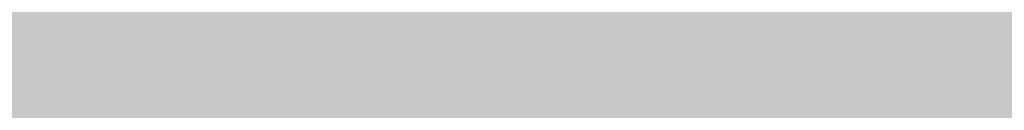
# Model space of a CAD drawing. Units: feet. Extents: x 3168 to 4724, y 827 to 1477.
# Tile 102 of 256: x 3277.376 to 3284.479, y 1098.344 to 1099.001. Entities that reach past the tile are written whole.
import ezdxf

# ---------------------------------------------------------------- set-up
doc = ezdxf.new("R2010")
doc.units = ezdxf.units.FT
doc.layers.add('A-ELEV', color=7, linetype='Continuous', lineweight=35)
doc.layers.add('A-ELEV-PATT', color=8, linetype='Continuous', lineweight=13)

msp = doc.modelspace()

# ---------------------------------------------------------------- hatches: boundary and pattern name
at = {"layer": 'A-ELEV-PATT'}
h = msp.add_hatch(color=256, dxfattribs=at)
h.dxf.hatch_style = 1
edge = h.paths.add_edge_path()
edge.add_ellipse((3552.9058, 979.2201), major_axis=(36.7449, 0), ratio=0.4848485, start_angle=0, end_angle=360)
edge = h.paths.add_edge_path()
edge.add_ellipse((3559.8916, 929.2523), major_axis=(36.7449, 0), ratio=0.4848485, start_angle=0, end_angle=360)
edge = h.paths.add_edge_path()
edge.add_line((3299.3168, 1198.6061), (3479.9167, 1198.6061))
edge.add_line((3479.9167, 1198.6061), (3479.9167, 1209.8686))
edge.add_spline(control_points=[(3479.9167, 1209.8686), (3464.3012, 1209.8686), (3448.6856, 1209.8686), (3410.9491, 1209.8686), (3388.8282, 1209.8686), (3355.6469, 1209.8686), (3344.5864, 1209.8686), (3327.9957, 1209.8686), (3322.4655, 1209.8686), (3314.1702, 1209.8686), (3311.4051, 1209.8686), (3307.2574, 1209.8686), (3305.8748, 1209.8686), (3303.801, 1209.8686), (3303.1097, 1209.8686), (3302.0728, 1209.8686), (3301.7272, 1209.8686), (3301.2087, 1209.8686), (3301.0359, 1209.8686), (3300.7767, 1209.8686), (3300.6903, 1209.8686), (3300.5606, 1209.8686), (3300.5174, 1209.8686), (3300.4526, 1209.8686), (3300.431, 1209.8686), (3300.3986, 1209.8686), (3300.3878, 1209.8686), (3300.3662, 1209.8686), (3300.3457, 1209.8686), (3300.3455, 1209.8686), (3300.3455, 1209.8686), (3300.3433, 1209.8686), (3300.3411, 1209.8686), (3300.3379, 1209.8686), (3300.3368, 1209.8686), (3300.3339, 1209.8686), (3300.3321, 1209.8686), (3300.3255, 1209.8686), (3300.3207, 1209.8686), (3300.3109, 1209.8686), (3300.306, 1209.8686), (3300.2905, 1209.8686), (3300.28, 1209.8686), (3300.2324, 1209.8688), (3300.1953, 1209.869), (3299.9511, 1209.8706), (3299.7448, 1209.8743), (3299.4368, 1209.8833), (3299.3344, 1209.8868), (3299.1811, 1209.8929), (3299.13, 1209.8951), (3298.6522, 1209.9168), (3298.2295, 1209.9457), (3297.6016, 1210.0024), (3297.3934, 1210.0235), (3297.0827, 1210.0583), (3296.9793, 1210.0705), (3296.293, 1210.1549), (3295.7181, 1210.2434), (3294.8687, 1210.3989), (3294.5877, 1210.4545), (3294.1693, 1210.5433), (3294.0304, 1210.5739), (3291.7071, 1211.1012), (3289.6536, 1211.8134), (3285.7763, 1213.564), (3283.9514, 1214.6035), (3280.5122, 1216.9801), (3278.8972, 1218.3176), (3276.3799, 1220.8295), (3275.416, 1221.9177), (3274.0393, 1223.7077), (3273.581, 1224.3495), (3273.1432, 1225.0163)], knot_values=[39.119033, 39.119033, 39.119033, 39.119033, 39.286353, 39.286353, 39.523379, 39.523379, 39.641892, 39.641892, 39.701148, 39.701148, 39.730777, 39.730777, 39.745591, 39.745591, 39.752998, 39.752998, 39.756701, 39.756701, 39.758553, 39.758553, 39.759479, 39.759479, 39.759942, 39.759942, 39.760173, 39.760173, 39.760289, 39.760289, 39.760405, 39.760405, 39.760463, 39.760463, 39.763389, 39.763389, 39.764851, 39.764851, 39.767304, 39.767304, 39.773825, 39.773825, 39.78057, 39.78057, 39.79477, 39.79477, 39.845194, 39.845194, 40.126715, 40.126715, 40.267476, 40.267476, 40.337856, 40.337856, 40.927023, 40.927023, 41.221606, 41.221606, 41.368898, 41.368898, 42.202622, 42.202622, 42.619485, 42.619485, 42.827916, 42.827916, 46.118323, 46.118323, 49.408731, 49.408731, 52.699139, 52.699139, 54.927489, 54.927489, 56.104228, 56.104228, 56.104228, 56.104228], weights=[1, 1, 1, 1, 1, 1, 1, 1, 1, 1, 1, 1, 1, 1, 1, 1, 1, 1, 1, 1, 1, 1, 1, 1, 1, 1, 1, 1, 1, 1, 1, 1, 1, 1, 1, 1, 1, 1, 1, 1, 1, 1, 1, 1, 1, 1, 1, 1, 1, 1, 1, 1, 1, 1, 1, 1, 1, 1, 1, 1, 1, 1, 1, 1, 1, 1, 1, 1, 1, 1, 1, 1, 1, 1], degree=3, periodic=0)
edge.add_line((3273.1432, 1225.0163), (3273.1432, 1099.0163))
edge.add_line((3273.1432, 1099.0163), (3299.3168, 1099.0163))
edge.add_line((3299.3168, 1099.0163), (3299.3168, 1198.6061))
edge = h.paths.add_edge_path()
edge.add_line((3304.7584, 1324.1581), (3479.9167, 1324.1581))
edge.add_line((3479.9167, 1324.1581), (3479.9167, 1335.7146))
edge.add_line((3479.9167, 1335.7146), (3269.1616, 1335.7146))
edge.add_spline(control_points=[(3269.1616, 1335.7146), (3264.0242, 1335.7146), (3258.3641, 1328.9582), (3259.2643, 1323.9003)], knot_values=[0, 0, 0, 0, 15.412191, 15.412191, 15.412191, 15.412191], degree=3, periodic=0)
edge.add_line((3259.2643, 1323.9003), (3265.5168, 1288.7691))
edge.add_line((3265.5168, 1288.7691), (3275.2651, 1261.5456))
edge.add_line((3275.2651, 1261.5456), (3304.7584, 1261.5456))
edge.add_line((3304.7584, 1261.5456), (3304.7584, 1324.1581))
h = msp.add_hatch(color=256, dxfattribs=at)
h.dxf.hatch_style = 1
h.paths.add_polyline_path([(3384.5252, 1099.0163), (3335.0292, 1099.0163), (3299.3168, 1099.0163), (3273.1432, 1099.0163), (3217.5654, 1099.0163), (3168.0693, 827.1163), (3335.0292, 827.1163)])

# ---------------------------------------------------------------- linework, layer by layer
at = {"layer": 'A-ELEV'}
msp.add_open_spline([(3808.5202, 1099.0163), (3808.5202, 1141.4132), (3808.5202, 1183.8102), (3808.5202, 1226.6353), (3808.5202, 1227.0636), (3808.5202, 1227.4918), (3811.4919, 1248.9947), (3814.4635, 1270.4975), (3817.4652, 1292.2176), (3817.4952, 1292.4348), (3817.5253, 1292.652), (3817.5728, 1310.1067), (3817.6203, 1327.5615), (3817.6679, 1345.0163), (3817.6679, 1345.458), (3817.6679, 1345.8996), (3817.6679, 1346.456), (3817.6679, 1346.5708), (3817.6679, 1346.7529), (3817.6679, 1346.8201), (3817.6679, 1346.9349), (3817.6679, 1346.9823), (3817.6679, 1347.0386), (3817.6679, 1347.0474), (3817.6679, 1347.0737), (3817.6679, 1347.0593), (3817.6679, 1347.0615), (3817.6679, 1347.0627), (3817.6679, 1347.066), (3817.6679, 1347.0683), (3817.6679, 1347.075), (3817.6679, 1347.0795), (3817.6678, 1347.0929), (3817.6678, 1347.1019), (3817.6678, 1347.1288), (3817.6677, 1347.1467), (3817.6674, 1347.2004), (3817.6672, 1347.2362), (3817.6661, 1347.3434), (3817.665, 1347.4147), (3817.6608, 1347.6281), (3817.6566, 1347.7697), (3817.64, 1348.1925), (3817.6235, 1348.4716), (3817.5591, 1349.3001), (3817.4961, 1349.8406), (3817.2554, 1351.4242), (3817.0263, 1352.4288), (3816.3069, 1354.8889), (3815.7437, 1356.2687), (3814.464, 1358.8192), (3813.7464, 1359.991), (3812.1958, 1362.1723), (3811.3622, 1363.1821), (3809.5888, 1365.069), (3808.6488, 1365.9461), (3806.6543, 1367.5796), (3805.5997, 1368.3362), (3803.3529, 1369.7223), (3802.1605, 1370.3524), (3799.6008, 1371.4536), (3798.2327, 1371.9255), (3795.2801, 1372.6346), (3793.6931, 1372.8721), (3791.8694, 1372.9265), (3791.7409, 1372.9292), (3791.3534, 1372.9341), (3791.0927, 1372.9329), (3790.3041, 1372.9151), (3789.7695, 1372.8842), (3789.2092, 1372.8302), (3789.1906, 1372.8284), (3789.1349, 1372.8229), (3789.0977, 1372.8191), (3789.0484, 1372.814), (3789.0364, 1372.8127), (3789.0003, 1372.8089), (3788.9761, 1372.8063), (3788.9494, 1372.8034), (3788.9468, 1372.8031), (3788.9426, 1372.8027), (3788.941, 1372.8025), (3788.9386, 1372.8022), (3788.9378, 1372.8021), (3788.9354, 1372.8019), (3788.8675, 1372.7944), (3788.7569, 1372.7822), (3788.7015, 1372.7761), (3788.5355, 1372.7579), (3788.4249, 1372.7457), (3788.0929, 1372.7092), (3787.8715, 1372.6848), (3787.2075, 1372.6118), (3786.7648, 1372.5631), (3785.4368, 1372.417), (3784.5515, 1372.3196), (3781.8954, 1372.0274), (3780.1247, 1371.8327), (3774.8126, 1371.2483), (3771.2713, 1370.8587), (3760.6471, 1369.69), (3753.5643, 1368.9109), (3732.316, 1366.5735), (3718.1504, 1365.0152), (3694.0068, 1362.3593), (3684.0287, 1361.2617), (3674.0506, 1360.1641), (3664.6007, 1360.1641), (3655.1508, 1360.1641), (3626.8011, 1360.1641), (3607.9013, 1360.1641), (3551.2019, 1360.1641), (3513.4023, 1360.1641), (3467.7252, 1360.1641), (3459.8476, 1360.1641), (3436.2149, 1360.1641), (3420.4597, 1360.1641), (3373.1943, 1360.1641), (3341.6839, 1360.1641), (3302.8482, 1360.1641), (3295.5227, 1360.1641), (3286.0383, 1360.1641), (3283.8794, 1360.1641), (3277.4026, 1360.1641), (3273.0848, 1360.1641), (3267.7329, 1360.1641), (3266.6988, 1360.1641), (3263.5965, 1360.1641), (3261.5284, 1360.1641), (3259.2369, 1360.1641), (3259.0137, 1360.1641), (3258.344, 1360.1641), (3257.8975, 1360.1641), (3257.431, 1360.1641), (3257.411, 1360.1641), (3257.3706, 1360.1641), (3257.3755, 1360.1641), (3257.3746, 1360.1641), (3257.3739, 1360.1641), (3257.372, 1360.1641), (3257.3706, 1360.1641), (3257.3667, 1360.1641), (3257.364, 1360.1641), (3257.3561, 1360.1641), (3257.3508, 1360.164), (3257.335, 1360.164), (3257.3244, 1360.164), (3257.2928, 1360.1639), (3257.2717, 1360.1638), (3257.2084, 1360.1634), (3257.1663, 1360.163), (3257.0402, 1360.1614), (3256.9563, 1360.1598), (3256.7055, 1360.1534), (3256.5392, 1360.147), (3256.0436, 1360.1219), (3255.7173, 1360.0971), (3254.7524, 1360.0005), (3254.128, 1359.9065), (3252.1801, 1359.5253), (3250.9416, 1359.144), (3248.6702, 1358.2433), (3247.6357, 1357.7238), (3245.7326, 1356.6035), (3244.8634, 1356.0021), (3243.2531, 1354.7429), (3242.512, 1354.0847), (3240.7511, 1352.3448), (3239.801, 1351.2296), (3238.0878, 1348.8724), (3237.3247, 1347.6304), (3235.9825, 1344.9716), (3235.4022, 1343.5549), (3234.5911, 1340.8155), (3234.3109, 1339.5435), (3233.9765, 1336.8026), (3233.9221, 1335.3309), (3234.1489, 1332.5913), (3234.3495, 1331.3672), (3234.7199, 1329.9994), (3234.7524, 1329.8834), (3234.8536, 1329.5348), (3234.9259, 1329.3017), (3235.0248, 1329.0026), (3235.0469, 1328.9369), (3235.0776, 1328.8472), (3235.0859, 1328.8232), (3235.1109, 1328.7511), (3235.1278, 1328.703), (3235.148, 1328.6462), (3235.1511, 1328.6376), (3235.1561, 1328.6235), (3235.1581, 1328.618), (3235.1602, 1328.612), (3235.1656, 1328.5969), (3235.1801, 1328.5565), (3235.1903, 1328.5281), (3235.2208, 1328.4429), (3235.2411, 1328.3862), (3235.3021, 1328.2159), (3235.3427, 1328.1023), (3235.4647, 1327.7617), (3235.546, 1327.5346), (3235.79, 1326.8534), (3235.9526, 1326.3992), (3236.4405, 1325.0367), (3236.7657, 1324.1284), (3237.7415, 1321.4034), (3238.392, 1319.5868), (3240.3435, 1314.1369), (3241.6445, 1310.5036), (3245.5476, 1299.6037), (3248.1496, 1292.3371), (3255.9557, 1270.5374), (3261.1598, 1256.0042), (3267.3876, 1238.612), (3268.4114, 1235.7529), (3269.5104, 1232.6839), (3269.5856, 1232.4739), (3269.7066, 1232.1359), (3269.7524, 1232.0079), (3269.8273, 1231.7987), (3269.8564, 1231.7176), (3269.9063, 1231.5781), (3269.9272, 1231.5198), (3269.9725, 1231.3934), (3269.9968, 1231.3254), (3270.0265, 1231.2425), (3270.0318, 1231.2277), (3270.0403, 1231.204), (3270.0392, 1231.207), (3270.0394, 1231.2066), (3270.0394, 1231.2064), (3270.0396, 1231.2058), (3270.0398, 1231.2055), (3270.0402, 1231.2043), (3270.0404, 1231.2036), (3270.0413, 1231.2013), (3270.0418, 1231.1998), (3270.0434, 1231.1953), (3270.0445, 1231.1922), (3270.0478, 1231.1832), (3270.0499, 1231.1771), (3270.0564, 1231.159), (3270.0608, 1231.147), (3270.0739, 1231.1108), (3270.0826, 1231.0867), (3270.1089, 1231.0144), (3270.1266, 1230.9663), (3270.1799, 1230.8225), (3270.2159, 1230.7269), (3270.3253, 1230.4415), (3270.4, 1230.2528), (3270.6292, 1229.6914), (3270.7889, 1229.3235), (3271.2865, 1228.2383), (3271.6431, 1227.5398), (3272.7759, 1225.5153), (3273.6142, 1224.2605), (3275.416, 1221.9177), (3276.3799, 1220.8295), (3278.8972, 1218.3176), (3280.5122, 1216.9801), (3283.9514, 1214.6035), (3285.7763, 1213.564), (3289.6536, 1211.8134), (3291.7071, 1211.1012), (3294.0304, 1210.5739), (3294.1693, 1210.5433), (3294.5877, 1210.4545), (3294.8687, 1210.3989), (3295.7181, 1210.2434), (3296.293, 1210.1549), (3296.9793, 1210.0705), (3297.0827, 1210.0583), (3297.3934, 1210.0235), (3297.6016, 1210.0024), (3298.2295, 1209.9457), (3298.6522, 1209.9168), (3299.13, 1209.8951), (3299.1811, 1209.8929), (3299.3344, 1209.8868), (3299.4368, 1209.8833), (3299.7448, 1209.8743), (3299.9511, 1209.8706), (3300.1953, 1209.869), (3300.2324, 1209.8688), (3300.28, 1209.8686), (3300.2905, 1209.8686), (3300.306, 1209.8686), (3300.3109, 1209.8686), (3300.3207, 1209.8686), (3300.3255, 1209.8686), (3300.3321, 1209.8686), (3300.3339, 1209.8686), (3300.3368, 1209.8686), (3300.3379, 1209.8686), (3300.3411, 1209.8686), (3300.3433, 1209.8686), (3300.3455, 1209.8686), (3300.3455, 1209.8686), (3300.3457, 1209.8686), (3300.3662, 1209.8686), (3300.3878, 1209.8686), (3300.3986, 1209.8686), (3300.431, 1209.8686), (3300.4526, 1209.8686), (3300.5174, 1209.8686), (3300.5606, 1209.8686), (3300.6903, 1209.8686), (3300.7767, 1209.8686), (3301.0359, 1209.8686), (3301.2087, 1209.8686), (3301.7272, 1209.8686), (3302.0728, 1209.8686), (3303.1097, 1209.8686), (3303.801, 1209.8686), (3305.8748, 1209.8686), (3307.2574, 1209.8686), (3311.4051, 1209.8686), (3314.1702, 1209.8686), (3322.4655, 1209.8686), (3327.9957, 1209.8686), (3344.5864, 1209.8686), (3355.6469, 1209.8686), (3388.8282, 1209.8686), (3410.9491, 1209.8686), (3477.3119, 1209.8686), (3521.5537, 1209.8686), (3566.8362, 1209.8686), (3567.8769, 1209.8686), (3570.999, 1209.8686), (3573.0804, 1209.8686), (3575.7814, 1209.8686), (3576.4009, 1209.8686), (3577.2958, 1209.8686), (3577.5712, 1209.8686), (3578.3971, 1209.8686), (3578.9478, 1209.8686), (3579.7565, 1209.8686), (3580.0145, 1209.8686), (3580.3427, 1209.8686), (3580.3269, 1209.8686), (3580.3272, 1209.8686), (3580.3273, 1209.8686), (3580.3278, 1209.8686), (3580.3281, 1209.8686), (3580.329, 1209.8686), (3580.3296, 1209.8686), (3580.3314, 1209.8686), (3580.3327, 1209.8686), (3580.3363, 1209.8686), (3580.3388, 1209.8686), (3580.3461, 1209.8686), (3580.351, 1209.8686), (3580.3657, 1209.8685), (3580.3754, 1209.8685), (3580.4048, 1209.8684), (3580.4244, 1209.8684), (3580.4832, 1209.8681), (3580.5224, 1209.8678), (3580.6404, 1209.8666), (3580.7192, 1209.8655), (3580.9563, 1209.8608), (3581.1152, 1209.8561), (3581.5942, 1209.8372), (3581.9164, 1209.8183), (3582.8899, 1209.7424), (3583.548, 1209.6662), (3585.5318, 1209.3606), (3586.8672, 1209.0539), (3589.4715, 1208.2525), (3590.7402, 1207.7579), (3591.9955, 1207.1588), (3592.0578, 1207.1287), (3592.2442, 1207.038), (3592.3677, 1206.9766), (3592.7353, 1206.7904), (3592.9768, 1206.6631), (3593.2445, 1206.5164), (3593.2747, 1206.4998), (3593.3651, 1206.4498), (3593.4251, 1206.4163), (3593.6043, 1206.3153), (3593.7227, 1206.2472), (3593.8572, 1206.1684), (3593.8744, 1206.1583), (3593.9257, 1206.128), (3593.9599, 1206.1078), (3594.0621, 1206.0469), (3594.1298, 1206.0061), (3594.2084, 1205.9582), (3594.2197, 1205.9513), (3594.2534, 1205.9307), (3594.2758, 1205.9169), (3594.343, 1205.8755), (3594.3876, 1205.8479), (3594.4336, 1205.819), (3594.4353, 1205.818), (3594.4402, 1205.8149), (3594.4435, 1205.8129), (3594.4471, 1205.8106), (3594.4475, 1205.8103), (3594.4487, 1205.8096), (3594.4495, 1205.8091), (3594.4504, 1205.8086), (3594.4505, 1205.8085), (3594.4506, 1205.8084), (3594.4674, 1205.7979), (3594.4933, 1205.7817), (3594.5062, 1205.7736), (3594.545, 1205.7492), (3594.5709, 1205.733), (3594.6485, 1205.6844), (3594.7002, 1205.652), (3594.8554, 1205.5547), (3594.9589, 1205.4898), (3595.2694, 1205.2953), (3595.4763, 1205.1656), (3596.0972, 1204.7765), (3596.5111, 1204.5171), (3597.7528, 1203.7388), (3598.5807, 1203.22), (3601.0642, 1201.6636), (3602.7198, 1200.6259), (3607.6868, 1197.513), (3610.9981, 1195.4377), (3620.932, 1189.2119), (3627.5546, 1185.0614), (3647.4225, 1172.6097), (3660.6678, 1164.3086), (3700.4035, 1139.4053), (3726.894, 1122.8031), (3757.2057, 1103.8061), (3761.027, 1101.4112), (3764.8482, 1099.0163), (3745.3283, 1099.0163), (3725.8083, 1099.0163), (3706.2884, 1099.0163), (3706.2884, 1108.4532), (3706.2884, 1117.8902), (3706.2884, 1127.3271), (3710.7508, 1127.3271), (3715.2131, 1127.3271), (3719.6755, 1127.3271)], degree=3, knots=[0, 0, 0, 0, 0.982037, 0.982037, 0.991957, 0.991957, 0.991957, 1.966522, 1.966522, 1.976367, 1.976367, 1.976367, 2.976367, 2.976367, 2.976367, 3.00169, 3.00169, 3.008272, 3.008272, 3.012129, 3.012129, 3.014851, 3.014851, 3.015353, 3.015353, 3.016359, 3.016359, 3.017365, 3.017365, 3.019376, 3.019376, 3.023398, 3.023398, 3.031442, 3.031442, 3.047531, 3.047531, 3.079708, 3.079708, 3.144063, 3.144063, 3.272772, 3.272772, 3.53019, 3.53019, 4.045026, 4.045026, 5.074698, 5.074698, 6.700878, 6.700878, 8.327058, 8.327058, 9.953238, 9.953238, 11.579418, 11.579418, 13.205598, 13.205598, 14.831778, 14.831778, 16.457958, 16.457958, 18.084138, 18.084138, 18.206872, 18.206872, 18.45234, 18.45234, 18.943275, 18.943275, 18.960093, 18.960093, 18.993729, 18.993729, 19.00461, 19.00461, 19.026374, 19.026374, 19.028737, 19.028737, 19.03018, 19.03018, 19.030897, 19.030897, 19.032332, 19.032332, 19.033766, 19.033766, 19.036636, 19.036636, 19.042374, 19.042374, 19.053851, 19.053851, 19.076805, 19.076805, 19.122714, 19.122714, 19.21453, 19.21453, 19.398163, 19.398163, 19.765429, 19.765429, 20.024128, 20.024128, 20.024128, 20.092031, 20.092031, 20.227836, 20.227836, 20.499446, 20.499446, 20.556051, 20.556051, 20.66926, 20.66926, 20.895678, 20.895678, 20.948316, 20.948316, 20.963829, 20.963829, 20.994855, 20.994855, 21.002285, 21.002285, 21.017146, 21.017146, 21.01875, 21.01875, 21.021959, 21.021959, 21.022102, 21.022102, 21.022249, 21.022249, 21.022708, 21.022708, 21.023627, 21.023627, 21.025464, 21.025464, 21.029138, 21.029138, 21.036486, 21.036486, 21.051183, 21.051183, 21.080575, 21.080575, 21.139361, 21.139361, 21.256932, 21.256932, 21.492073, 21.492073, 21.962356, 21.962356, 23.01002, 23.01002, 24.057684, 24.057684, 25.105348, 25.105348, 26.153011, 26.153011, 27.776787, 27.776787, 29.400562, 29.400562, 31.024337, 31.024337, 32.278801, 32.278801, 33.533265, 33.533265, 34.467568, 34.467568, 34.553971, 34.553971, 34.726776, 34.726776, 34.775309, 34.775309, 34.793079, 34.793079, 34.82862, 34.82862, 34.834979, 34.834979, 34.839039, 34.839039, 34.839411, 34.839411, 34.840285, 34.840285, 34.842034, 34.842034, 34.845531, 34.845531, 34.852525, 34.852525, 34.866512, 34.866512, 34.894488, 34.894488, 34.950439, 34.950439, 35.062342, 35.062342, 35.286147, 35.286147, 35.733758, 35.733758, 35.821815, 35.821815, 35.828283, 35.828283, 35.832225, 35.832225, 35.834724, 35.834724, 35.836521, 35.836521, 35.838617, 35.838617, 35.839073, 35.839073, 35.839345, 35.839345, 35.839617, 35.839617, 35.840161, 35.840161, 35.841249, 35.841249, 35.843425, 35.843425, 35.847778, 35.847778, 35.856482, 35.856482, 35.873891, 35.873891, 35.908709, 35.908709, 35.978345, 35.978345, 36.117617, 36.117617, 36.396161, 36.396161, 36.953248, 36.953248, 38.067423, 38.067423, 40.295772, 40.295772, 42.524122, 42.524122, 45.81453, 45.81453, 49.104937, 49.104937, 52.395345, 52.395345, 52.603776, 52.603776, 53.020639, 53.020639, 53.854363, 53.854363, 54.001655, 54.001655, 54.296238, 54.296238, 54.885405, 54.885405, 54.955785, 54.955785, 55.096546, 55.096546, 55.378067, 55.378067, 55.42849, 55.42849, 55.442691, 55.442691, 55.449436, 55.449436, 55.455957, 55.455957, 55.458409, 55.458409, 55.459872, 55.459872, 55.462798, 55.462798, 55.462856, 55.462856, 55.462972, 55.462972, 55.463088, 55.463088, 55.463319, 55.463319, 55.463782, 55.463782, 55.464708, 55.464708, 55.46656, 55.46656, 55.470263, 55.470263, 55.47767, 55.47767, 55.492484, 55.492484, 55.522112, 55.522112, 55.581369, 55.581369, 55.699882, 55.699882, 55.936907, 55.936907, 56.410959, 56.410959, 56.42211, 56.42211, 56.444413, 56.444413, 56.451051, 56.451051, 56.454001, 56.454001, 56.459901, 56.459901, 56.462666, 56.462666, 56.463418, 56.463418, 56.464171, 56.464171, 56.465675, 56.465675, 56.468684, 56.468684, 56.474702, 56.474702, 56.486738, 56.486738, 56.51081, 56.51081, 56.558955, 56.558955, 56.655243, 56.655243, 56.847821, 56.847821, 57.232975, 57.232975, 58.003284, 58.003284, 59.543901, 59.543901, 62.625137, 62.625137, 68.787607, 68.787607, 74.950078, 74.950078, 75.27336, 75.27336, 75.919923, 75.919923, 77.213051, 77.213051, 77.377769, 77.377769, 77.707206, 77.707206, 78.366079, 78.366079, 78.462532, 78.462532, 78.655436, 78.655436, 79.041245, 79.041245, 79.105735, 79.105735, 79.234714, 79.234714, 79.492672, 79.492672, 79.502197, 79.502197, 79.521249, 79.521249, 79.523534, 79.523534, 79.528103, 79.528103, 79.528682, 79.528682, 79.528885, 79.528885, 79.529089, 79.529089, 79.529495, 79.529495, 79.530308, 79.530308, 79.531935, 79.531935, 79.535187, 79.535187, 79.541693, 79.541693, 79.554704, 79.554704, 79.580725, 79.580725, 79.632769, 79.632769, 79.736856, 79.736856, 79.94503, 79.94503, 80.361377, 80.361377, 80.421435, 80.421435, 80.421435, 81.421435, 81.421435, 81.421435, 82.421435, 82.421435, 82.421435, 83.421435, 83.421435, 83.421435, 83.421435], dxfattribs=at)

doc.saveas('drawing.dxf')
